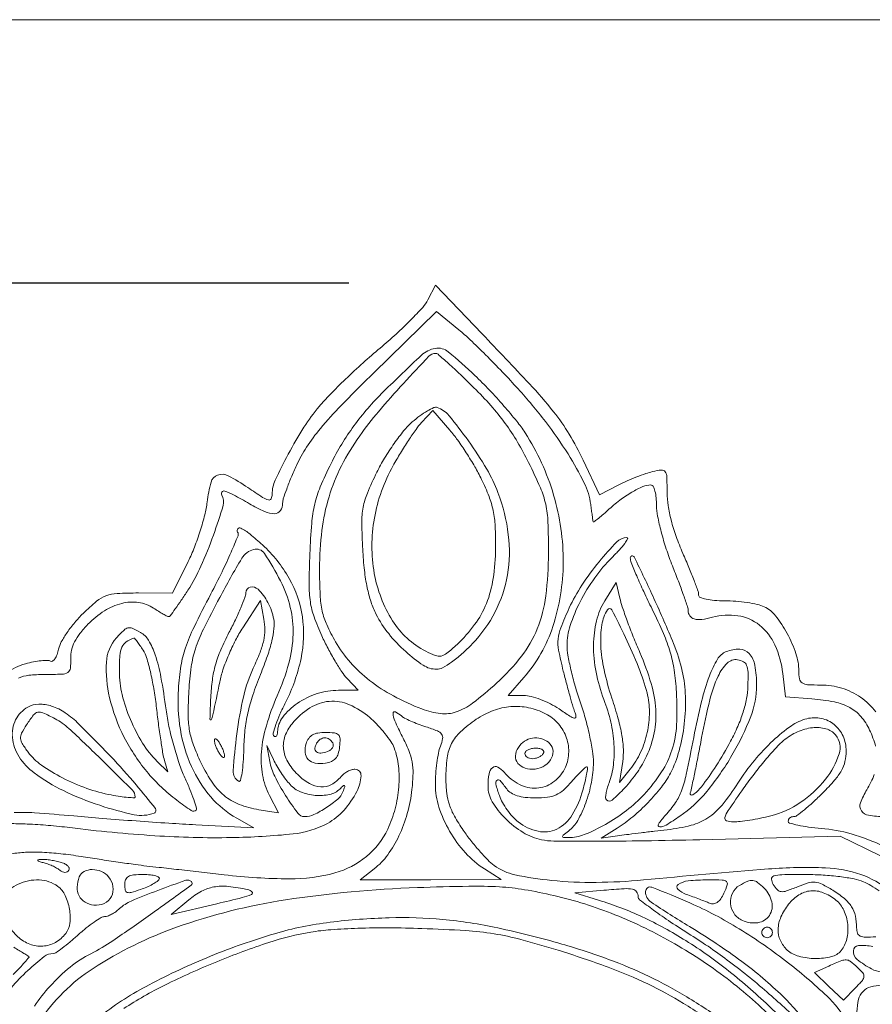
# Model space of a CAD drawing. Units: inches. Extents: x 2656 to 9931, y 1941 to 3068.
# Tile 40 of 46: x 2842.88 to 2854.27, y 2981.19 to 2994.35. Entities that reach past the tile are written whole.
import ezdxf

# ---------------------------------------------------------------- set-up
doc = ezdxf.new("R2010")
doc.units = ezdxf.units.IN
for name, color, linetype, lineweight in [('A-ANNO-DIMS', 2, 'Continuous', 18), ('A-ELEV-FNSH', 8, 'Continuous', 13), ('A-ELEV-ORN', 8, 'Continuous', 13)]:
    doc.layers.add(name, color=color, linetype=linetype, lineweight=lineweight)
doc.styles.get("Standard").update_dxf_attribs({"font": 'arial.ttf'})
doc.dimstyles.new('ISO-25', dxfattribs={"dimtxt": 6, "dimasz": 2.5, "dimexe": 1.25, "dimexo": 0.625, "dimtad": 1, "dimdec": 0, "dimlunit": 3, "dimtxsty": 'Standard', "dimcen": 2.5, "dimadec": 0, "dimazin": 0, "dimtfac": 1, "dimtdec": 0, "dimtmove": 0, "dimatfit": 3, "dimfxl": 1, "dimarcsym": 0})

# ---------------------------------------------------------------- blocks, each defined once
blk = doc.blocks.new('*D152')
at = {"layer": 'A-ANNO-DIMS', "color": 0, "lineweight": -2, "transparency": 16777216}
for p, q in [((2847.28, 2990.828), (2707.323, 2990.828)), ((2708.573, 2988.328), (2708.573, 2952.971)), ((2847.248, 2950.471), (2707.323, 2950.471))]:
    blk.add_line(p, q, dxfattribs=at)
at = {"layer": 'A-ANNO-DIMS', "color": 0, "transparency": 16777216}
for points in [[(2708.156, 2988.328), (2708.989, 2988.328), (2708.573, 2990.828)], [(2708.156, 2952.971), (2708.989, 2952.971), (2708.573, 2950.471)]]:
    blk.add_solid(points, dxfattribs=at)
at = {"layer": 'Defpoints', "color": 0, "transparency": 16777216}
for p in [(2847.905, 2990.828), (2708.573, 2950.471), (2847.873, 2950.471)]:
    blk.add_point(p, dxfattribs=at)
at = {"layer": 'A-ANNO-DIMS', "color": 0, "transparency": 16777216, "insert": (2704.843, 2970.649), "char_height": 6, "attachment_point": 5, "rotation": 90}
blk.add_mtext('3\'-4 1/2"', dxfattribs=at)
blk = doc.blocks.new('*D153')
at = {"layer": 'A-ANNO-DIMS', "color": 0, "lineweight": -2, "transparency": 16777216}
for p, q in [((2826.64, 2993.722), (2826.64, 2703.709)), ((2829.546, 2956.424), (2829.546, 2703.709)), ((2824.14, 2704.959), (2821.64, 2704.959)), ((2826.64, 2704.959), (2829.546, 2704.959)), ((2832.046, 2704.959), (2851.745, 2704.959))]:
    blk.add_line(p, q, dxfattribs=at)
at = {"layer": 'A-ANNO-DIMS', "color": 0, "transparency": 16777216}
for points in [[(2824.14, 2705.376), (2824.14, 2704.543), (2826.64, 2704.959)], [(2832.046, 2705.376), (2832.046, 2704.543), (2829.546, 2704.959)]]:
    blk.add_solid(points, dxfattribs=at)
at = {"layer": 'Defpoints', "color": 0, "transparency": 16777216}
for p in [(2826.64, 2994.347), (2829.546, 2957.049), (2829.546, 2704.959)]:
    blk.add_point(p, dxfattribs=at)
at = {"layer": 'A-ANNO-DIMS', "color": 0, "transparency": 16777216, "insert": (2843.145, 2708.65), "char_height": 6, "attachment_point": 5}
blk.add_mtext('0\'-3"', dxfattribs=at)
blk = doc.blocks.new('*D154')
at = {"layer": 'A-ANNO-DIMS', "color": 0, "lineweight": -2, "transparency": 16777216}
for p, q in [((2708.573, 2996.847), (2708.573, 2999.347)), ((2826.015, 2994.347), (2707.323, 2994.347)), ((2708.573, 2994.347), (2708.573, 2990.828)), ((2847.28, 2990.828), (2707.323, 2990.828)), ((2708.573, 2988.328), (2708.573, 2954.647))]:
    blk.add_line(p, q, dxfattribs=at)
at = {"layer": 'A-ANNO-DIMS', "color": 0, "transparency": 16777216}
for points in [[(2708.156, 2996.847), (2708.989, 2996.847), (2708.573, 2994.347)], [(2708.156, 2988.328), (2708.989, 2988.328), (2708.573, 2990.828)]]:
    blk.add_solid(points, dxfattribs=at)
at = {"layer": 'Defpoints', "color": 0, "transparency": 16777216}
for p in [(2826.64, 2994.347), (2708.573, 2990.828), (2847.905, 2990.828)]:
    blk.add_point(p, dxfattribs=at)
at = {"layer": 'A-ANNO-DIMS', "color": 0, "transparency": 16777216, "insert": (2704.843, 2970.237), "char_height": 6, "attachment_point": 5, "rotation": 90}
blk.add_mtext('0\'-3 1/2"', dxfattribs=at)

msp = doc.modelspace()

# ---------------------------------------------------------------- linework, layer by layer
at = {"layer": 'A-ELEV-FNSH'}
msp.add_lwpolyline([(2826.64, 2994.347), (2868.226, 2994.347), (2868.226, 2892.035), (2826.64, 2892.035)], close=True, dxfattribs=at)
at = {"layer": 'A-ELEV-ORN'}
for points in [[(2854.315, 2985.099, 0.078135), (2854.113, 2985.294, 0.079077), (2853.862, 2985.416, 0.074196), (2853.581, 2985.458, -0.014444), (2853.405, 2985.463, -0.128754), (2853.332, 2985.487, -0.206552), (2853.297, 2985.539, -0.046553), (2853.287, 2985.647, 0.081788), (2853.249, 2985.878, 0.042113), (2853.132, 2986.146, 0.041941), (2852.978, 2986.382, 0.120789), (2852.825, 2986.503, 0.050427), (2852.733, 2986.534, 0.018265), (2852.597, 2986.56, 0.017897), (2852.445, 2986.578, 0.020342), (2852.299, 2986.584, -0.018674), (2852.16, 2986.589, -0.035131), (2852.048, 2986.605, -0.042536), (2851.971, 2986.629, -0.305397), (2851.95, 2986.66, 0.085772), (2851.942, 2986.71, 0.004985), (2851.888, 2986.855, 0.007447), (2851.82, 2987.027, 0.005403), (2851.739, 2987.217, -0.017471), (2851.649, 2987.443, -0.022274), (2851.583, 2987.659, -0.024666), (2851.542, 2987.856, -0.039017), (2851.528, 2988.027, 0.008441), (2851.525, 2988.241, 0.142371), (2851.503, 2988.308, 0.273929), (2851.454, 2988.331, 0.034912), (2851.335, 2988.31, 0.024588), (2851.243, 2988.283, 0.010575), (2851.122, 2988.238, 0.010434), (2850.996, 2988.185, 0.013571), (2850.883, 2988.131), (2850.624, 2987.998), (2850.407, 2988.462, 0.026394), (2850.221, 2988.808, 0.032728), (2850.012, 2989.109, 0.019173), (2849.69, 2989.482, 0.003433), (2849.057, 2990.151), (2848.435, 2990.799), (2848.335, 2990.605, -0.064322), (2848.264, 2990.503, -0.01162), (2848.105, 2990.336, -0.012355), (2847.909, 2990.147, -0.010908), (2847.695, 2989.96, 0.00918), (2847.469, 2989.763, 0.007525), (2847.234, 2989.545, 0.007613), (2847.024, 2989.337, 0.019853), (2846.881, 2989.18, 0.032915), (2846.679, 2988.903, 0.018495), (2846.469, 2988.543, 0.015337), (2846.295, 2988.194, 0.10597), (2846.254, 2988.008, -0.116612), (2846.239, 2987.947, -0.354776), (2846.203, 2987.931, -0.077717), (2846.127, 2987.965, -0.005231), (2845.93, 2988.096, 0.027818), (2845.667, 2988.253, 0.209245), (2845.526, 2988.264, 0.245289), (2845.437, 2988.168, 0.037684), (2845.385, 2987.903, -0.03191), (2845.354, 2987.732, -0.0157), (2845.293, 2987.518, -0.01551), (2845.216, 2987.3, -0.021792), (2845.133, 2987.11), (2844.924, 2986.686), (2844.467, 2986.688, 0.013726), (2844.183, 2986.681, 0.075832), (2844.034, 2986.65, 0.085147), (2843.909, 2986.578, 0.019712), (2843.728, 2986.414, 0.025371), (2843.617, 2986.294, 0.023836), (2843.516, 2986.161, 0.024569), (2843.438, 2986.035, 0.071714), (2843.402, 2985.939, -0.032608), (2843.381, 2985.865, -0.059736), (2843.352, 2985.809, -0.094985), (2843.322, 2985.778, -0.298499), (2843.295, 2985.777, 0.144064), (2843.255, 2985.788, 0.021126), (2843.17, 2985.783, 0.022408), (2843.067, 2985.768, 0.017548), (2842.958, 2985.742, 0.091949), (2842.702, 2985.62, 0.038622)], [(2842.866, 2985.551, -0.083292), (2843.002, 2985.588, -0.025328), (2843.215, 2985.599, 0.00912), (2843.445, 2985.603, 0.128792), (2843.524, 2985.627, 0.230001), (2843.559, 2985.682, 0.036545), (2843.565, 2985.813, -0.063476), (2843.576, 2985.925, -0.05995), (2843.615, 2986.034, -0.049883), (2843.686, 2986.146, -0.026445), (2843.794, 2986.27, -0.057798), (2844.014, 2986.449, -0.082041), (2844.245, 2986.549, -0.095324), (2844.469, 2986.561, -0.11109), (2844.669, 2986.486, 0.007454), (2844.737, 2986.443, 0.010398), (2844.8, 2986.406, 0.007107), (2844.853, 2986.377, 0.120632), (2844.872, 2986.373, 0.235905), (2844.89, 2986.382, 0.003736), (2844.96, 2986.476, 0.008958), (2845.039, 2986.59, 0.005707), (2845.128, 2986.724, 0.036676), (2845.302, 2987.046, 0.020464), (2845.469, 2987.459, 0.013319), (2845.599, 2987.859, 0.213754), (2845.581, 2987.997, -0.305446), (2845.583, 2988.037, -0.321124), (2845.62, 2988.05, -0.047856), (2845.739, 2987.999, -0.008628), (2845.949, 2987.881, 0.025918), (2846.153, 2987.776, 0.110206), (2846.287, 2987.747, 0.24323), (2846.363, 2987.788, 0.152107), (2846.394, 2987.887, -0.078541), (2846.403, 2987.947, -0.008908), (2846.448, 2988.076, -0.010604), (2846.507, 2988.23, -0.008438), (2846.578, 2988.393, -0.040004), (2846.712, 2988.635, -0.027614), (2846.899, 2988.886, -0.019052), (2847.176, 2989.193, -0.006251), (2847.606, 2989.624), (2848.45, 2990.448), (2848.749, 2990.203, -0.01845), (2848.897, 2990.072, -0.006117), (2849.105, 2989.87, -0.006081), (2849.329, 2989.64, -0.006877), (2849.539, 2989.414, -0.019396), (2849.903, 2988.978, -0.023978), (2850.205, 2988.545, -0.025885), (2850.422, 2988.156, -0.081827), (2850.508, 2987.871, 0.000371), (2850.518, 2987.794, 0.000496), (2850.528, 2987.723, 0.000342), (2850.536, 2987.664, 0.00521), (2850.539, 2987.643, 0.548711), (2850.549, 2987.639, 0.013408), (2850.599, 2987.674, 0.016834), (2850.662, 2987.726, 0.009167), (2850.737, 2987.793, -0.025193), (2850.895, 2987.926, -0.02965), (2851.057, 2988.034, -0.031965), (2851.205, 2988.109, -0.101207), (2851.313, 2988.131, -0.284785), (2851.342, 2988.113, -0.049006), (2851.366, 2988.05, -0.040655), (2851.382, 2987.961, -0.025665), (2851.388, 2987.855, 0.049109), (2851.402, 2987.714, 0.015173), (2851.45, 2987.505, 0.015015), (2851.518, 2987.274, 0.015963), (2851.599, 2987.052, -0.004381), (2851.679, 2986.845, -0.006165), (2851.748, 2986.659, -0.003777), (2851.802, 2986.501, -0.081071), (2851.81, 2986.453, 0.155966), (2851.832, 2986.382, 0.172026), (2851.891, 2986.341, 0.10107), (2851.991, 2986.334, 0.034921), (2852.134, 2986.363, -0.105391), (2852.473, 2986.384, -0.132014), (2852.762, 2986.259, -0.119243), (2852.969, 2985.993, -0.076479), (2853.074, 2985.614), (2853.111, 2985.3), (2853.462, 2985.273, -0.029523), (2853.762, 2985.232, -0.074901), (2853.968, 2985.158, -0.093016), (2854.116, 2985.038, -0.065621), (2854.233, 2984.857, -0.044451), (2854.313, 2984.64, -0.078218)], [(2854.424, 2983.306, 0.034451), (2853.986, 2983.469, 0.051823), (2853.586, 2983.543, -0.012852), (2853.418, 2983.561, -0.020808), (2853.275, 2983.586, -0.016013), (2853.165, 2983.614, -0.33473), (2853.146, 2983.639, -0.118163), (2853.152, 2983.662, -0.100614), (2853.167, 2983.682, -0.092537), (2853.191, 2983.695, -0.082719), (2853.218, 2983.7, 0.160905), (2853.261, 2983.714, 0.011177), (2853.362, 2983.792, 0.014973), (2853.479, 2983.894, 0.010663), (2853.605, 2984.015, 0.016588), (2853.766, 2984.187, 0.052031), (2853.857, 2984.316, 0.071324), (2853.904, 2984.437, 0.056637), (2853.92, 2984.576, 0.103225), (2853.878, 2984.775, 0.118359), (2853.761, 2984.93, 0.1216), (2853.589, 2985.012, 0.112975), (2853.394, 2985.008, 0.091427), (2853.188, 2984.914, 0.035379), (2852.943, 2984.715, 0.032673), (2852.695, 2984.451, 0.029758), (2852.475, 2984.149, -0.028189), (2852.263, 2983.855, -0.076789), (2852.074, 2983.684, -0.082317), (2851.85, 2983.584, -0.035894), (2851.528, 2983.525, 0.001697), (2851.362, 2983.506, 0.001346), (2851.183, 2983.484, 0.00136), (2851.017, 2983.463, 0.003403), (2850.895, 2983.447), (2850.649, 2983.412), (2850.86, 2983.546, 0.032786), (2851.07, 2983.699, 0.026073), (2851.276, 2983.89, 0.026722), (2851.452, 2984.093, 0.046509), (2851.573, 2984.281, 0.053502), (2851.689, 2984.58, 0.036945), (2851.758, 2984.938, 0.036528), (2851.773, 2985.307, 0.047498), (2851.731, 2985.643, 0.042706), (2851.615, 2986.012, 0.009719), (2851.353, 2986.613, 0.007724), (2851.088, 2987.169, 0.786926), (2851.037, 2987.157, 0.098595), (2851.049, 2987.096, 0.005676), (2851.122, 2986.917, 0.008467), (2851.216, 2986.706, 0.00611), (2851.328, 2986.473, -0.012354), (2851.48, 2986.145, -0.031365), (2851.57, 2985.898, -0.035368), (2851.622, 2985.659, -0.019934), (2851.653, 2985.365, -0.029859), (2851.655, 2984.925, -0.062769), (2851.593, 2984.589, -0.068214), (2851.455, 2984.297, -0.041404), (2851.22, 2983.995, -0.043392), (2850.988, 2983.783, -0.033937), (2850.704, 2983.595, -0.034654), (2850.423, 2983.46, -0.09505), (2850.208, 2983.419, -0.016241), (2850.143, 2983.421, -0.40699), (2850.132, 2983.433, -0.217056), (2850.142, 2983.452, -0.007438), (2850.211, 2983.507, 0.104056), (2850.334, 2983.648, 0.040712), (2850.442, 2983.884, 0.0392), (2850.518, 2984.158, 0.04772), (2850.544, 2984.424, 0.039125), (2850.532, 2984.576, 0.014351), (2850.492, 2984.788, 0.014125), (2850.435, 2985.019, 0.016453), (2850.368, 2985.234, -0.01367), (2850.3, 2985.445, -0.013019), (2850.244, 2985.663, -0.01308), (2850.203, 2985.858, -0.044292), (2850.192, 2985.987, -0.079543), (2850.235, 2986.253, -0.038926), (2850.367, 2986.571, -0.037036), (2850.562, 2986.89, -0.041614), (2850.794, 2987.164, 0.012038), (2850.891, 2987.265, 0.024408), (2850.962, 2987.35, 0.032837), (2851.001, 2987.411, 0.572992), (2850.992, 2987.428, 0.203102), (2850.857, 2987.371, 0.020739), (2850.621, 2987.106, 0.026278), (2850.389, 2986.791, 0.038243), (2850.222, 2986.489, 0.01216), (2850.108, 2986.222, 0.071457), (2850.073, 2986.075, 0.072281), (2850.08, 2985.924, 0.012602), (2850.142, 2985.645, 0.003624), (2850.188, 2985.47, 0.004047), (2850.233, 2985.302, 0.003736), (2850.275, 2985.159, 0.021333), (2850.301, 2985.085, -0.093964), (2850.311, 2985.032, -0.486856), (2850.291, 2985.016, -0.082498), (2850.231, 2985.042, -0.006579), (2850.086, 2985.138, 0.031762), (2849.969, 2985.207, 0.026558), (2849.837, 2985.265, 0.027385), (2849.711, 2985.305, 0.063462), (2849.612, 2985.318), (2849.404, 2985.318), (2849.615, 2985.558, 0.101844), (2850.003, 2986.241, 0.077512), (2850.141, 2987.092, 0.072839), (2850.013, 2987.996, 0.072078), (2849.632, 2988.829, 0.026422), (2849.52, 2988.983, 0.010022), (2849.349, 2989.186, 0.009893), (2849.154, 2989.4, 0.01192), (2848.962, 2989.593, 0.018391), (2848.606, 2989.91, 0.219576), (2848.432, 2989.956, 0.145576), (2848.247, 2989.864, 0.006907), (2847.743, 2989.379, 0.01889), (2847.531, 2989.153, 0.021022), (2847.345, 2988.92, 0.021463), (2847.183, 2988.676, 0.021586), (2847.042, 2988.42, 0.014989), (2846.897, 2988.105, 0.041973), (2846.822, 2987.874, 0.03764), (2846.782, 2987.619, 0.010219), (2846.757, 2987.213, 0.008108), (2846.747, 2986.804, 0.038176), (2846.764, 2986.569, 0.050177), (2846.813, 2986.371, 0.020973), (2846.917, 2986.115, 0.013565), (2847, 2985.947, 0.012733), (2847.094, 2985.779, 0.012815), (2847.184, 2985.635, 0.042128), (2847.254, 2985.546), (2847.403, 2985.388), (2847.14, 2985.388, 0.07865), (2846.855, 2985.343, 0.071598), (2846.588, 2985.212, 0.079818), (2846.395, 2985.028, 0.158524), (2846.326, 2984.831, -0.047162), (2846.322, 2984.796, -0.134812), (2846.31, 2984.775, -0.251455), (2846.295, 2984.769, -0.15697), (2846.277, 2984.778, -0.271092), (2846.267, 2984.814, -0.01545), (2846.303, 2984.929, -0.020165), (2846.358, 2985.069, -0.01311), (2846.433, 2985.225, 0.065004), (2846.639, 2985.812, 0.088793), (2846.657, 2986.371, 0.092884), (2846.481, 2986.882, 0.078127), (2846.124, 2987.331, 0.016395), (2845.958, 2987.474, 0.049956), (2845.834, 2987.555, 0.368564), (2845.795, 2987.546, 0.306498), (2845.793, 2987.502, -0.23943), (2845.798, 2987.452, -0.005733), (2845.705, 2987.232, -0.011318), (2845.585, 2986.972, -0.007294), (2845.435, 2986.676, 0.007423), (2845.21, 2986.232, 0.031468), (2845.097, 2985.957, 0.042853), (2845.036, 2985.714, 0.022925), (2845.002, 2985.405, 0.056615), (2845.028, 2984.863, 0.065886), (2845.177, 2984.369, 0.071367), (2845.435, 2983.964, 0.08766), (2845.781, 2983.679), (2846.007, 2983.552), (2845.233, 2983.592, -0.003395), (2844.876, 2983.612, -0.00184), (2844.436, 2983.642, -0.001832), (2843.989, 2983.676, -0.002895), (2843.606, 2983.709, 0.005241), (2843.08, 2983.751, 0.032074), (2842.808, 2983.753, 0.046774)], [(2842.742, 2983.607, -0.010086), (2842.983, 2983.601, -0.010454), (2843.264, 2983.583, -0.009794), (2843.55, 2983.553, 0.014603), (2844.689, 2983.445, 0.020573), (2845.709, 2983.42, 0.021554), (2846.535, 2983.469, 0.098726), (2846.992, 2983.61, 0.086544), (2847.211, 2983.783, 0.064842), (2847.385, 2984.037, 0.105005), (2847.441, 2984.247, 0.429394), (2847.36, 2984.333, 0.076994), (2847.314, 2984.326, 0.044443), (2847.262, 2984.304, 0.043169), (2847.213, 2984.273, 0.055175), (2847.174, 2984.235, -0.094539), (2847.045, 2984.129, -0.137453), (2846.903, 2984.096, -0.121204), (2846.751, 2984.141, -0.064485), (2846.595, 2984.261, -0.062539), (2846.462, 2984.433, -0.106068), (2846.405, 2984.604, -0.115654), (2846.425, 2984.774, -0.084243), (2846.519, 2984.939, -0.078947), (2846.757, 2985.152, -0.123459), (2847.016, 2985.24, -0.122999), (2847.287, 2985.195, -0.078015), (2847.559, 2985.023, -0.023138), (2847.662, 2984.924, -0.02043), (2847.759, 2984.812, -0.020932), (2847.839, 2984.703, -0.056713), (2847.883, 2984.619, -0.065298), (2847.941, 2984.376, -0.046), (2847.945, 2984.096, -0.044024), (2847.896, 2983.805, -0.046139), (2847.797, 2983.533, -0.111372), (2847.513, 2983.167, -0.104185), (2847.092, 2982.948, -0.070935), (2846.484, 2982.868, -0.025816), (2845.614, 2982.922, 0.000041), (2845.311, 2982.957, 0.000041), (2845.008, 2982.992, 0.00004), (2844.743, 2983.022, 0.000159), (2844.58, 2983.04, -0.005888), (2844.426, 2983.06, -0.001908), (2844.198, 2983.092, -0.001902), (2843.945, 2983.13, -0.002136), (2843.701, 2983.168, 0.013188), (2843.43, 2983.204, 0.017307), (2843.181, 2983.223, 0.019272), (2842.96, 2983.223, 0.031038), (2842.772, 2983.203, -0.002177)], [(2854.502, 2982.71, 0.090302), (2854.115, 2982.926, 0.071489), (2853.644, 2983.015, 0.030983), (2852.881, 2983.001, 0.003778), (2851.212, 2982.854, -0.021814), (2850.58, 2982.821, -0.026279), (2849.987, 2982.847, -0.027515), (2849.496, 2982.923, -0.109001), (2849.219, 2983.048, -0.039008), (2849.134, 2983.122, -0.013678), (2849.023, 2983.242, -0.013486), (2848.908, 2983.38, -0.015368), (2848.806, 2983.519, -0.021273), (2848.689, 2983.706, -0.047989), (2848.621, 2983.858, -0.052132), (2848.586, 2984.013, -0.029551), (2848.574, 2984.205, -0.032073), (2848.592, 2984.486, -0.085895), (2848.651, 2984.678, -0.089345), (2848.77, 2984.834, -0.036649), (2848.979, 2985, -0.05968), (2849.206, 2985.117, -0.069858), (2849.442, 2985.17, -0.071671), (2849.679, 2985.155, -0.067725), (2849.906, 2985.074, -0.096375), (2850.077, 2984.939, -0.095623), (2850.185, 2984.75, -0.097447), (2850.213, 2984.537, -0.104526), (2850.158, 2984.335, -0.120644), (2850, 2984.154, -0.141327), (2849.786, 2984.08, -0.132721), (2849.555, 2984.13, -0.100833), (2849.352, 2984.293, 0.099524), (2849.267, 2984.362, 0.306948), (2849.198, 2984.354, 0.175194), (2849.15, 2984.27, 0.041792), (2849.137, 2984.109, 0.134004), (2849.194, 2983.899, 0.062873), (2849.368, 2983.674, 0.060359), (2849.605, 2983.488, 0.086765), (2849.852, 2983.391, 0.047774), (2850.015, 2983.374, 0.002239), (2850.569, 2983.372, 0.003679), (2851.228, 2983.377, 0.002634), (2851.964, 2983.392), (2853.842, 2983.44), (2854.371, 2983.182, -0.01869)], [(2854.296, 2984.264, -0.046304), (2854.196, 2984.059, 0.047957), (2854.111, 2983.884, 0.239863), (2854.123, 2983.779, 0.210398), (2854.218, 2983.718, 0.03751), (2854.433, 2983.701, -0.076239)], [(2854.317, 2982.096, -0.017844), (2854.177, 2982.089, -0.111032), (2854.108, 2982.103, -0.203959), (2854.072, 2982.142, -0.084493), (2854.06, 2982.213, 0.053126), (2854.043, 2982.372, 0.088219), (2853.992, 2982.496, 0.078617), (2853.897, 2982.605, 0.034796), (2853.741, 2982.717, 0.021635), (2853.599, 2982.796, 0.093332), (2853.506, 2982.823, 0.097889), (2853.412, 2982.814, 0.025071), (2853.268, 2982.762, -0.014374), (2853.124, 2982.707, -0.11002), (2853.053, 2982.698, -0.177871), (2853.001, 2982.723, -0.052147), (2852.946, 2982.794, -0.128312), (2852.923, 2982.866, -0.345735), (2852.953, 2982.907, -0.067863), (2853.061, 2982.924, -0.004017), (2853.394, 2982.926, -0.016087), (2853.614, 2982.919, -0.015606), (2853.835, 2982.898, -0.015762), (2854.028, 2982.867, -0.053298), (2854.15, 2982.83, -0.033959), (2854.25, 2982.779, -0.019972), (2854.361, 2982.707, -0.019921)], [(2842.766, 2981.414, -0.024978), (2842.99, 2981.643, -0.020758), (2843.209, 2981.829, -0.166976), (2843.332, 2981.871, 0.152907), (2843.366, 2981.882, 0.009354), (2843.451, 2981.944, 0.013229), (2843.552, 2982.023, 0.009364), (2843.66, 2982.117, -0.013871), (2843.77, 2982.212, -0.01812), (2843.877, 2982.291, -0.015858), (2843.968, 2982.351, -0.136675), (2844.015, 2982.364, 0.09123), (2844.054, 2982.371, 0.031745), (2844.108, 2982.395, 0.030285), (2844.164, 2982.43, 0.030912), (2844.215, 2982.471, -0.082228), (2844.372, 2982.572, -0.011888), (2844.725, 2982.714, -0.006268), (2845.099, 2982.849, -0.287599), (2845.175, 2982.832, -0.460996), (2845.172, 2982.784, -0.001493), (2844.628, 2982.392, -0.006319), (2844.125, 2982.041, -0.032689), (2843.833, 2981.869, 0.054333), (2843.557, 2981.69, 0.037267), (2843.287, 2981.434, 0.03621), (2843.078, 2981.168, 0.154288)], [(2843.141, 2980.957, -0.10364), (2843.864, 2981.673, -0.058168), (2844.978, 2982.222, -0.047464), (2846.434, 2982.588, -0.029352), (2848.193, 2982.752, -0.004362), (2848.88, 2982.77, -0.01877), (2849.289, 2982.762, -0.026526), (2849.624, 2982.724, -0.016022), (2850.016, 2982.646, -0.038715), (2850.832, 2982.389, -0.034771), (2851.63, 2982.001, -0.034471), (2852.373, 2981.502, -0.036376), (2853.026, 2980.915, 0.00697)], [(2853.43, 2980.888, 0.039762), (2853.073, 2981.299, 0.035403), (2852.526, 2981.765, 0.022219), (2851.827, 2982.232, -0.010114), (2851.315, 2982.557, -0.257227), (2851.241, 2982.699, -0.51849), (2851.326, 2982.756, -0.012975), (2851.834, 2982.547, -0.034146), (2852.492, 2982.201, -0.0272), (2853.15, 2981.743, -0.027027), (2853.697, 2981.268, -0.092556), (2853.968, 2980.885, 0.014479)], [(2852.297, 2980.956, 0.020948), (2851.793, 2981.291, 0.02459), (2851.288, 2981.564, 0.02374), (2850.745, 2981.793, 0.017347), (2850.122, 2981.998, 0.017713), (2849.266, 2982.213, 0.029402), (2848.532, 2982.326, 0.031017), (2847.817, 2982.349, 0.022786), (2847.027, 2982.289, 0.041752), (2846.286, 2982.136, 0.024654), (2845.432, 2981.836, 0.024644), (2844.611, 2981.454, 0.041345), (2843.97, 2981.045, 0.012422)], [(2844.271, 2981.135, -0.0302), (2844.821, 2981.45, -0.01769), (2845.514, 2981.762, -0.017702), (2846.211, 2982.019, -0.037526), (2846.77, 2982.157, -0.023556), (2847.037, 2982.189, -0.010004), (2847.398, 2982.208, -0.009217), (2847.812, 2982.214, -0.007701), (2848.253, 2982.205, -0.007144), (2848.836, 2982.177, -0.023875), (2849.217, 2982.134, -0.025809), (2849.576, 2982.058, -0.009462), (2850.075, 2981.914, -0.013133), (2850.741, 2981.688, -0.023644), (2851.272, 2981.464, -0.025775), (2851.747, 2981.205, -0.019692), (2852.24, 2980.876, -0.007963)], [(2842.804, 2981.955, 0.000076), (2842.874, 2981.911, 0.000108), (2842.936, 2981.873, 0.000061), (2842.989, 2981.84, 0.001532), (2843.003, 2981.831, -0.455409), (2843.005, 2981.819, -0.005577), (2842.951, 2981.755, -0.011717), (2842.882, 2981.678, -0.006865), (2842.795, 2981.589, -0.020091)], [(2854.528, 2981.626, -0.173005), (2854.26, 2981.665, -0.048254), (2854.067, 2981.792, -0.240913), (2854.016, 2981.906, -0.374645), (2854.084, 2981.976, -0.070536), (2854.276, 2981.965, 0.042314)], [(2854.063, 2981.092, -0.053592), (2854.085, 2981.259, -0.136805), (2854.145, 2981.365, -0.127241), (2854.248, 2981.426, -0.071275), (2854.394, 2981.446, -0.065833)]]:
    msp.add_lwpolyline(points, format="xyb", dxfattribs=at)
for points in [[(2848.949, 2989.431, -0.017705), (2849.174, 2989.192, -0.022163), (2849.365, 2988.954, -0.022708), (2849.53, 2988.705, -0.020336), (2849.679, 2988.432, -0.012444), (2849.836, 2988.093, -0.048338), (2849.907, 2987.873, -0.044828), (2849.937, 2987.635, -0.009686), (2849.944, 2987.22, -0.031328), (2849.907, 2986.648, -0.063117), (2849.794, 2986.211, -0.069293), (2849.584, 2985.842, -0.04557), (2849.251, 2985.483, -0.019387), (2848.931, 2985.217, -0.080794), (2848.71, 2985.098, -0.114651), (2848.505, 2985.077, -0.060196), (2848.254, 2985.139, -0.031621), (2847.874, 2985.313, -0.042292), (2847.556, 2985.519, -0.046038), (2847.299, 2985.76, -0.051489), (2847.101, 2986.035, -0.022207), (2846.983, 2986.265, -0.053988), (2846.922, 2986.445, -0.043412), (2846.895, 2986.657, -0.010375), (2846.887, 2987.012, -0.030913), (2846.918, 2987.524, -0.042839), (2847.013, 2987.973, -0.044516), (2847.179, 2988.386, -0.037558), (2847.424, 2988.789, -0.019818), (2847.674, 2989.11, -0.010653), (2848.006, 2989.487, -0.004218), (2848.347, 2989.851, -0.20536), (2848.437, 2989.889, -0.181057), (2848.469, 2989.877, -0.00329), (2848.608, 2989.755, -0.007702), (2848.768, 2989.607, -0.005012)], [(2848.125, 2988.973, 0.041366), (2848.013, 2988.857, 0.017676), (2847.883, 2988.685, 0.017347), (2847.756, 2988.491, 0.021841), (2847.652, 2988.302, 0.015479), (2847.526, 2988.023, 0.053533), (2847.469, 2987.833, 0.048234), (2847.451, 2987.625, 0.010916), (2847.463, 2987.271, 0.013767), (2847.486, 2986.991, 0.023714), (2847.523, 2986.759, 0.028229), (2847.575, 2986.566, 0.039754), (2847.644, 2986.401, 0.05001), (2847.81, 2986.145, 0.03921), (2848.037, 2985.904, 0.039535), (2848.272, 2985.722, 0.145915), (2848.449, 2985.669, 0.125304), (2848.53, 2985.69, 0.029667), (2848.649, 2985.765, 0.027356), (2848.786, 2985.873, 0.019289), (2848.927, 2986.009, 0.073793), (2849.232, 2986.436, 0.076247), (2849.396, 2986.929, 0.072747), (2849.408, 2987.467, 0.058947), (2849.27, 2988.029, 0.044539), (2849.12, 2988.343, 0.021074), (2848.874, 2988.72, 0.016594), (2848.614, 2989.059, 0.142094), (2848.458, 2989.166, 0.186611), (2848.412, 2989.164, 0.027261), (2848.327, 2989.121, 0.027725), (2848.227, 2989.055, 0.020547)], [(2849.05, 2988.206, -0.021855), (2849.15, 2987.979, -0.042029), (2849.205, 2987.789, -0.037924), (2849.232, 2987.58, -0.014668), (2849.238, 2987.287, -0.03482), (2849.205, 2986.88, -0.058125), (2849.116, 2986.549, -0.062666), (2848.958, 2986.265, -0.048569), (2848.723, 2986, -0.016192), (2848.587, 2985.883, -0.117547), (2848.511, 2985.846, -0.144734), (2848.433, 2985.852, -0.028801), (2848.304, 2985.91, -0.134355), (2847.861, 2986.318, -0.09671), (2847.618, 2986.95, -0.087319), (2847.619, 2987.686, -0.083772), (2847.869, 2988.389, -0.009605), (2847.968, 2988.558, -0.009005), (2848.075, 2988.727, -0.009012), (2848.175, 2988.873, -0.030344), (2848.248, 2988.964), (2848.398, 2989.128), (2848.628, 2988.862, -0.023773), (2848.73, 2988.733, -0.011854), (2848.847, 2988.56, -0.011739), (2848.96, 2988.375, -0.01693)], [(2846.365, 2986.85, -0.05862), (2846.496, 2986.496, -0.066947), (2846.534, 2986.136, -0.060176), (2846.476, 2985.75, -0.036203), (2846.321, 2985.312, 0.031452), (2846.176, 2984.915, 0.052381), (2846.111, 2984.565, 0.062293), (2846.125, 2984.257, 0.076873), (2846.217, 2983.984), (2846.338, 2983.75), (2846.077, 2983.792, -0.053112), (2845.813, 2983.864, -0.08112), (2845.609, 2983.985, -0.07403), (2845.442, 2984.173, -0.037264), (2845.288, 2984.452, -0.02111), (2845.194, 2984.683, -0.046993), (2845.147, 2984.867, -0.040967), (2845.132, 2985.071, -0.012781), (2845.142, 2985.378, -0.01958), (2845.174, 2985.704, -0.045505), (2845.229, 2985.944, -0.035232), (2845.335, 2986.203, -0.007951), (2845.553, 2986.627, -0.011569), (2845.849, 2987.152, -0.193973), (2846.005, 2987.27, -0.324163), (2846.151, 2987.216, -0.027798)], [(2845.902, 2986.69, -0.090133), (2845.89, 2986.628, -0.009811), (2845.836, 2986.491, -0.011764), (2845.763, 2986.329, -0.009238), (2845.677, 2986.158, 0.019456), (2845.568, 2985.929, 0.032634), (2845.497, 2985.728, 0.034126), (2845.455, 2985.526, 0.023904), (2845.434, 2985.295, 0.003033), (2845.423, 2985, 0.7785), (2845.439, 2984.995, 0.08097), (2845.463, 2985.059, 0.000964), (2845.553, 2985.5, -0.033342), (2845.597, 2985.663, -0.017451), (2845.673, 2985.86, -0.017281), (2845.765, 2986.057, -0.025301), (2845.861, 2986.223), (2846.096, 2986.588), (2846.143, 2986.337, -0.047851), (2846.156, 2986.193, -0.051834), (2846.141, 2986.054, -0.040393), (2846.092, 2985.894, -0.016103), (2846.002, 2985.684, 0.053301), (2845.874, 2985.312, 0.024063), (2845.782, 2984.804, 0.015985), (2845.734, 2984.311, 0.278337), (2845.805, 2984.174, 0.503517), (2845.83, 2984.183, 0.02371), (2845.851, 2984.284, 0.023184), (2845.867, 2984.427, 0.01246), (2845.875, 2984.604, -0.022882), (2845.891, 2984.853, -0.027681), (2845.929, 2985.085, -0.025678), (2845.996, 2985.324, -0.015771), (2846.098, 2985.599, 0.012836), (2846.191, 2985.847, 0.025315), (2846.25, 2986.049, 0.031987), (2846.278, 2986.212, 0.071965), (2846.274, 2986.338, 0.072982), (2846.198, 2986.559, 0.08496), (2846.065, 2986.737, 0.256007), (2845.96, 2986.765, 0.344476)], [(2850.697, 2986.584, 0.080947), (2850.586, 2986.317, 0.055842), (2850.546, 2985.991, 0.05064), (2850.579, 2985.632, 0.042649), (2850.684, 2985.264, -0.034798), (2850.776, 2984.962, -0.040702), (2850.818, 2984.666, -0.044215), (2850.811, 2984.39, -0.062064), (2850.753, 2984.152, 0.022148), (2850.728, 2984.076, 0.030665), (2850.713, 2984.007, 0.031217), (2850.707, 2983.95, 0.206016), (2850.718, 2983.924, 0.393222), (2850.795, 2983.922, 0.02864), (2850.962, 2984.084, 0.03328), (2851.132, 2984.295, 0.044428), (2851.255, 2984.509, 0.058439), (2851.356, 2984.819, 0.065899), (2851.377, 2985.131, 0.056234), (2851.315, 2985.477, 0.029068), (2851.166, 2985.891, -0.006369), (2851.077, 2986.104, -0.006544), (2850.995, 2986.318, -0.00636), (2850.929, 2986.505, -0.027359), (2850.897, 2986.619), (2850.85, 2986.83)], [(2851.26, 2985.353, -0.065214), (2851.293, 2985.097, -0.054073), (2851.263, 2984.823, -0.053572), (2851.175, 2984.559, -0.061101), (2851.035, 2984.333), (2850.894, 2984.157), (2850.935, 2984.438, 0.046822), (2850.944, 2984.601, 0.032179), (2850.925, 2984.784, 0.02531), (2850.875, 2985.005, 0.012096), (2850.791, 2985.282, -0.025663), (2850.687, 2985.66, -0.04185), (2850.643, 2985.989, -0.051154), (2850.657, 2986.261, -0.099954), (2850.732, 2986.464, -0.581878), (2850.791, 2986.462, -0.009223), (2850.973, 2986.095, -0.01655), (2851.147, 2985.695, -0.029412)], [(2844.174, 2986.087, 0.172154), (2844.04, 2985.765, 0.071457), (2844.083, 2985.289, 0.061299), (2844.278, 2984.759, 0.055784), (2844.602, 2984.274, 0.030445), (2844.774, 2984.093, 0.024242), (2844.979, 2983.92, 0.016218), (2845.174, 2983.781, 0.357434), (2845.238, 2983.787, 0.279023), (2845.245, 2983.814, 0.008257), (2845.207, 2983.927, 0.014252), (2845.155, 2984.063, 0.009073), (2845.088, 2984.219, -0.026189), (2845.013, 2984.408, -0.013812), (2844.939, 2984.65, -0.013706), (2844.876, 2984.903, -0.020542), (2844.837, 2985.126, 0.011953), (2844.768, 2985.565, 0.034959), (2844.692, 2985.861, 0.052725), (2844.604, 2986.056, 0.138047), (2844.494, 2986.162, 0.019078), (2844.382, 2986.217, 0.16317), (2844.327, 2986.222, 0.139123), (2844.276, 2986.193, 0.012602)], [(2844.53, 2985.925, -0.072616), (2844.577, 2985.825, -0.01487), (2844.627, 2985.637, -0.015364), (2844.672, 2985.412, -0.0139), (2844.706, 2985.178, 0.004271), (2844.734, 2984.945, 0.004996), (2844.766, 2984.724, 0.004436), (2844.795, 2984.538, 0.030229), (2844.817, 2984.448), (2844.861, 2984.298), (2844.718, 2984.438, -0.058565), (2844.524, 2984.682, -0.04017), (2844.361, 2984.996, -0.04022), (2844.25, 2985.331, -0.059423), (2844.213, 2985.639, -0.016262), (2844.22, 2985.851, -0.085274), (2844.247, 2985.964, -0.138013), (2844.304, 2986.034, -0.070648), (2844.405, 2986.086, -0.31492), (2844.415, 2986.083, -0.006173), (2844.449, 2986.041, -0.012411), (2844.487, 2985.988, -0.007711)], [(2852.318, 2985.904, 0.165424), (2852.202, 2985.804, 0.042576), (2852.094, 2985.579, 0.03085), (2851.989, 2985.24, 0.01187), (2851.884, 2984.758, -0.004218), (2851.784, 2984.263, -0.035106), (2851.721, 2984.043, -0.064087), (2851.641, 2983.889, -0.03207), (2851.506, 2983.718, 0.032911), (2851.413, 2983.6, 0.585663), (2851.43, 2983.565, 0.151652), (2851.514, 2983.586, 0.013225), (2851.7, 2983.707, 0.070327), (2852.057, 2984.035, 0.039471), (2852.395, 2984.52, 0.039624), (2852.645, 2985.036, 0.0932), (2852.724, 2985.455, 0.04232), (2852.701, 2985.722, 0.142454), (2852.625, 2985.879, 0.207068), (2852.498, 2985.937, 0.10069)], [(2852.607, 2985.445, -0.03794), (2852.589, 2985.276, -0.029771), (2852.544, 2985.096, -0.027125), (2852.473, 2984.906, -0.020589), (2852.376, 2984.707, -0.017432), (2852.183, 2984.378, -0.024362), (2851.987, 2984.1, -0.072868), (2851.874, 2983.991, -0.707506), (2851.838, 2984.016, 0.015846), (2851.859, 2984.103, 0.001992), (2851.899, 2984.291, 0.002341), (2851.944, 2984.516, 0.001941), (2851.99, 2984.755, -0.013973), (2852.099, 2985.259, -0.04764), (2852.21, 2985.576, -0.087896), (2852.331, 2985.75, -0.236693), (2852.47, 2985.796, -0.091197), (2852.548, 2985.77, -0.174607), (2852.591, 2985.721, -0.088585), (2852.609, 2985.631, -0.013427)], [(2842.99, 2985.163, 0.150682), (2842.828, 2984.993, 0.140741), (2842.784, 2984.756, 0.118986), (2842.873, 2984.5, 0.09113), (2843.076, 2984.283, 0.047148), (2843.466, 2984.047, 0.03133), (2843.951, 2983.851, 0.029184), (2844.412, 2983.726, 0.144139), (2844.677, 2983.747, 0.505083), (2844.694, 2983.808, 0.008532), (2844.437, 2984.124, 0.014242), (2844.098, 2984.503, 0.008445), (2843.673, 2984.937, 0.045857), (2843.491, 2985.087, 0.069431), (2843.308, 2985.177, 0.084935), (2843.137, 2985.203, 0.123164)], [(2843.355, 2985.008, -0.067699), (2843.539, 2984.878, -0.005874), (2843.955, 2984.481, -0.002811), (2844.387, 2984.054, -0.198928), (2844.424, 2983.963, -0.426413), (2844.413, 2983.951, -0.01023), (2844.33, 2983.957, -0.016119), (2844.227, 2983.968, -0.009459), (2844.104, 2983.989, -0.03958), (2843.78, 2984.077, -0.03311), (2843.453, 2984.218, -0.03433), (2843.172, 2984.388, -0.079387), (2842.996, 2984.56, -0.020214), (2842.915, 2984.677, -0.12579), (2842.893, 2984.746, -0.13582), (2842.908, 2984.814, -0.025008), (2842.974, 2984.927, -0.018278), (2843.067, 2985.058, -0.179078), (2843.124, 2985.094, -0.159807), (2843.193, 2985.087, -0.013801)], [(2847.98, 2985.045, 0.068851), (2848.021, 2985.016, 0.013641), (2848.104, 2984.977, 0.014209), (2848.203, 2984.936, 0.012792), (2848.307, 2984.9, -0.016005), (2848.46, 2984.845, -0.140058), (2848.517, 2984.802, -0.211156), (2848.53, 2984.744, -0.043005), (2848.501, 2984.641, 0.042878), (2848.475, 2984.55, 0.015421), (2848.453, 2984.418, 0.015166), (2848.438, 2984.271, 0.017397), (2848.434, 2984.129, 0.078277), (2848.481, 2983.826, 0.053409), (2848.624, 2983.506, 0.052411), (2848.835, 2983.216, 0.066536), (2849.088, 2983.002), (2849.313, 2982.858), (2848.371, 2982.857), (2847.43, 2982.856), (2847.617, 2983.003, 0.068721), (2847.797, 2983.189, 0.046574), (2847.947, 2983.443, 0.043279), (2848.059, 2983.742, 0.039834), (2848.121, 2984.064, 0.022084), (2848.135, 2984.274, 0.051136), (2848.123, 2984.431, 0.051223), (2848.079, 2984.582, 0.022226), (2847.991, 2984.773, -0.011889), (2847.892, 2984.978, -0.096537), (2847.868, 2985.08, -0.566329), (2847.899, 2985.1, -0.074818)], [(2853.778, 2984.791, -0.25773), (2853.826, 2984.538, -0.090134), (2853.644, 2984.2, -0.074143), (2853.307, 2983.888, -0.0883), (2852.912, 2983.71, -0.011429), (2852.776, 2983.679, -0.010081), (2852.633, 2983.653, -0.01018), (2852.504, 2983.635, -0.029989), (2852.414, 2983.63, -0.084474), (2852.322, 2983.645, -0.40285), (2852.3, 2983.688, -0.075006), (2852.345, 2983.781, -0.003121), (2852.553, 2984.083, -0.011443), (2852.69, 2984.269, -0.010427), (2852.84, 2984.456, -0.010498), (2852.98, 2984.616, -0.032945), (2853.084, 2984.716, -0.067963), (2853.27, 2984.833, -0.080185), (2853.47, 2984.888, -0.094887), (2853.65, 2984.874, -0.153097)], [(2846.708, 2984.678, 0.095719), (2846.694, 2984.555, 0.177301), (2846.735, 2984.465, 0.16002), (2846.828, 2984.416, 0.075231), (2846.966, 2984.415, 0.065371), (2847.045, 2984.437, 0.113861), (2847.1, 2984.477, 0.10333), (2847.135, 2984.54, 0.047341), (2847.155, 2984.632, 0.032384), (2847.16, 2984.741, 0.191818), (2847.138, 2984.793, 0.175052), (2847.086, 2984.819, 0.02616), (2846.966, 2984.825, 0.040287), (2846.865, 2984.817, 0.090069), (2846.793, 2984.792, 0.108516), (2846.742, 2984.746, 0.077838)], [(2847.062, 2984.684, -0.153283), (2847.07, 2984.654, -0.123144), (2847.06, 2984.621, -0.097937), (2847.033, 2984.592, -0.067341), (2846.993, 2984.57, -0.067736), (2846.906, 2984.549, -0.188422), (2846.846, 2984.566, -0.261672), (2846.825, 2984.613, -0.113371), (2846.848, 2984.68, -0.098738), (2846.897, 2984.733, -0.152164), (2846.956, 2984.752, -0.155876), (2847.014, 2984.735, -0.104938)], [(2849.56, 2984.65, 0.120997), (2849.506, 2984.541, 0.17779), (2849.521, 2984.435, 0.166411), (2849.602, 2984.36, 0.105001), (2849.73, 2984.333, 0.11812), (2849.867, 2984.366, 0.125643), (2849.971, 2984.457, 0.154147), (2850.006, 2984.572, 0.195996), (2849.964, 2984.674, 0.107231), (2849.87, 2984.734, 0.104431), (2849.758, 2984.751, 0.103241), (2849.649, 2984.721, 0.102471)], [(2845.482, 2984.72, 0.067616), (2845.486, 2984.686, 0.024967), (2845.502, 2984.639, 0.024204), (2845.524, 2984.59, 0.026766), (2845.55, 2984.544, 0.027796), (2845.576, 2984.508, 0.102785), (2845.598, 2984.49, 0.335455), (2845.612, 2984.492, 0.190341), (2845.618, 2984.509, 0.067616), (2845.613, 2984.543, 0.024967), (2845.598, 2984.589, 0.024204), (2845.576, 2984.639, 0.026766), (2845.55, 2984.685, 0.027796), (2845.524, 2984.721, 0.102785), (2845.502, 2984.739, 0.335455), (2845.488, 2984.736, 0.190341)], [(2846.494, 2984.128, 0.114674), (2846.634, 2984.031, 0.072561), (2846.829, 2983.984, 0.07473), (2847.022, 2983.996, 0.144021), (2847.158, 2984.069, -0.010392), (2847.205, 2984.115, -0.390187), (2847.219, 2984.115, -0.296739), (2847.223, 2984.099, -0.008211), (2847.198, 2984.031, -0.125375), (2847.13, 2983.935, -0.032964), (2846.978, 2983.821, -0.033465), (2846.811, 2983.727, -0.111069), (2846.688, 2983.7, -0.237289), (2846.595, 2983.747, -0.018951), (2846.433, 2983.982, -0.025659), (2846.289, 2984.239, -0.068375), (2846.222, 2984.438), (2846.182, 2984.649), (2846.271, 2984.462, 0.021971), (2846.315, 2984.38, 0.013532), (2846.373, 2984.287, 0.013562), (2846.436, 2984.198, 0.023552)], [(2849.875, 2984.544, -0.08825), (2849.851, 2984.517, -0.053305), (2849.815, 2984.494, -0.051278), (2849.773, 2984.479, -0.061875), (2849.731, 2984.474, -0.067639), (2849.692, 2984.479, -0.08433), (2849.659, 2984.494, -0.09965), (2849.637, 2984.517, -0.142666), (2849.629, 2984.544, -0.195654), (2849.64, 2984.571, -0.086673), (2849.672, 2984.594, -0.066561), (2849.719, 2984.609, -0.0466), (2849.774, 2984.614, -0.047867), (2849.827, 2984.609, -0.104212), (2849.864, 2984.594, -0.181468), (2849.88, 2984.571, -0.202618)], [(2850.404, 2984.055, -0.070868), (2850.262, 2983.724, -0.142621), (2850.054, 2983.534, -0.171173), (2849.805, 2983.504, -0.112091), (2849.54, 2983.629, -0.04338), (2849.467, 2983.698, -0.027284), (2849.393, 2983.79, -0.027315), (2849.329, 2983.89, -0.044304), (2849.288, 2983.981, -0.01773), (2849.241, 2984.133, -0.279933), (2849.256, 2984.184, -0.419522), (2849.297, 2984.181, -0.02352), (2849.386, 2984.071, 0.095953), (2849.444, 2984.017, 0.062749), (2849.526, 2983.979, 0.049607), (2849.634, 2983.957, 0.026969), (2849.77, 2983.949, 0.030515), (2849.931, 2983.959, 0.07475), (2850.045, 2983.991, 0.076493), (2850.143, 2984.054, 0.033118), (2850.252, 2984.165, -0.009074), (2850.325, 2984.246, -0.014868), (2850.39, 2984.312, -0.008551), (2850.445, 2984.363, -0.355115), (2850.46, 2984.364, -0.279189), (2850.467, 2984.348, -0.006538), (2850.453, 2984.266, -0.012561), (2850.432, 2984.168, -0.007953)], [(2843.421, 2983.093, -0.044106), (2843.479, 2983.072, -0.077101), (2843.521, 2983.044, -0.118075), (2843.541, 2983.014, -0.231054), (2843.538, 2982.985, -0.118725), (2843.516, 2982.963, -0.137872), (2843.487, 2982.955, -0.110622), (2843.453, 2982.963, -0.059296), (2843.416, 2982.986, 0.04364), (2843.375, 2983.013, 0.020287), (2843.317, 2983.043, 0.019919), (2843.253, 2983.068, 0.026211), (2843.194, 2983.086, -0.015792), (2843.143, 2983.1, -0.142678), (2843.124, 2983.113, -0.54732), (2843.128, 2983.123, -0.049857), (2843.158, 2983.128, -0.035484), (2843.21, 2983.128, -0.014647), (2843.279, 2983.121, -0.014406), (2843.353, 2983.109, -0.017979)], [(2844.07, 2982.894, -0.135667), (2844.128, 2982.765, -0.159637), (2844.107, 2982.633, -0.162671), (2844.011, 2982.541, -0.141286), (2843.874, 2982.518, -0.105321), (2843.755, 2982.558, -0.139981), (2843.676, 2982.641, -0.129176), (2843.65, 2982.758, -0.083137), (2843.678, 2982.895, -0.184777), (2843.742, 2982.967, -0.119411), (2843.852, 2982.993, -0.104438), (2843.974, 2982.967, -0.115499)], [(2844.745, 2982.863, -0.107608), (2844.717, 2982.834, -0.021914), (2844.656, 2982.796, -0.022157), (2844.579, 2982.759, -0.019191), (2844.495, 2982.726, -0.014382), (2844.372, 2982.687, -0.143386), (2844.319, 2982.687, -0.270702), (2844.292, 2982.717, -0.05545), (2844.284, 2982.789, -0.09425), (2844.297, 2982.857, -0.17529), (2844.334, 2982.899, -0.103586), (2844.404, 2982.921, -0.021985), (2844.534, 2982.926, -0.024047), (2844.627, 2982.922, -0.048936), (2844.699, 2982.908, -0.086446), (2844.741, 2982.887, -0.390075)], [(2843.39, 2982.768, -0.122481), (2843.49, 2982.647, -0.068858), (2843.547, 2982.464, -0.069741), (2843.553, 2982.276, -0.137892), (2843.497, 2982.139, -0.099844), (2843.36, 2982.02, -0.111741), (2843.192, 2981.97, -0.109476), (2843.017, 2981.996, -0.092694), (2842.858, 2982.095, -0.030108), (2842.785, 2982.169, -0.024708), (2842.717, 2982.256, -0.025392), (2842.663, 2982.342, -0.058376), (2842.633, 2982.413, -0.219842), (2842.666, 2982.628, -0.137448), (2842.863, 2982.797, -0.118866), (2843.143, 2982.855, -0.152619)], [(2845.928, 2982.725, -0.142351), (2845.984, 2982.694, -0.52366), (2845.978, 2982.661, -0.046126), (2845.854, 2982.618, -0.003756), (2845.517, 2982.536), (2844.904, 2982.392), (2845.139, 2982.587, -0.048979), (2845.311, 2982.703, -0.081146), (2845.475, 2982.76, -0.069614), (2845.667, 2982.767, -0.027738)], [(2852.288, 2982.677, -0.039546), (2852.245, 2982.6, -0.094648), (2852.199, 2982.554, -0.131667), (2852.15, 2982.536, -0.118349), (2852.096, 2982.544, 0.004767), (2852.04, 2982.566, 0.001676), (2851.959, 2982.597, 0.001664), (2851.87, 2982.63, 0.001949), (2851.785, 2982.661, -0.09908), (2851.673, 2982.73, -0.484847), (2851.677, 2982.793, -0.124471), (2851.811, 2982.842, -0.023719), (2852.072, 2982.855, -0.007897), (2852.266, 2982.853, -0.166438), (2852.32, 2982.833, -0.310843), (2852.332, 2982.79, -0.026295)], [(2852.824, 2982.745, -0.140164), (2852.927, 2982.56, -0.207169), (2852.895, 2982.38, -0.211953), (2852.742, 2982.283, -0.144526), (2852.535, 2982.312, -0.133745), (2852.424, 2982.404, -0.132485), (2852.375, 2982.54, -0.137045), (2852.401, 2982.679, -0.146835), (2852.495, 2982.78, -0.027347), (2852.605, 2982.836, -0.13142), (2852.674, 2982.847, -0.139092), (2852.737, 2982.822, -0.031997)], [(2851.141, 2982.631, 0.234084), (2851.162, 2982.589, 0.005273), (2851.348, 2982.45, 0.010754), (2851.575, 2982.292, 0.006932), (2851.845, 2982.118, -0.022141), (2852.364, 2981.76, -0.017515), (2852.893, 2981.33, -0.010813), (2853.352, 2980.911, -0.205251), (2853.427, 2980.736, -0.610427), (2853.405, 2980.725, -0.012924), (2853.278, 2980.821, -0.01531), (2853.113, 2980.961, -0.008092), (2852.917, 2981.143, 0.023749), (2852.355, 2981.635, 0.02817), (2851.779, 2982.043, 0.029993), (2851.196, 2982.361, 0.036248), (2850.614, 2982.584), (2850.297, 2982.68), (2850.684, 2982.716, -0.006356), (2850.954, 2982.737, -0.06236), (2851.067, 2982.73, -0.194631), (2851.121, 2982.696, -0.155959)], [(2853.783, 2982.586, -0.115772), (2853.889, 2982.448, -0.081816), (2853.941, 2982.26, -0.082026), (2853.929, 2982.065, -0.117515), (2853.852, 2981.91, -0.160977), (2853.723, 2981.829, -0.06248), (2853.509, 2981.804, -0.061343), (2853.289, 2981.834, -0.120718), (2853.134, 2981.917, -0.104097), (2853.041, 2982.045, -0.112553), (2853.011, 2982.195, -0.097841), (2853.049, 2982.36, -0.062182), (2853.151, 2982.53, -0.085196), (2853.29, 2982.655, -0.119698), (2853.447, 2982.708, -0.116006), (2853.614, 2982.684, -0.076773)], [(2852.935, 2982.153, -0.099038), (2852.93, 2982.126, -0.097945), (2852.914, 2982.103, -0.097945), (2852.891, 2982.088, -0.099038), (2852.865, 2982.082, -0.099038), (2852.838, 2982.088, -0.097945), (2852.815, 2982.103, -0.097945), (2852.8, 2982.126, -0.099038), (2852.794, 2982.153, -0.099038), (2852.8, 2982.179, -0.097945), (2852.815, 2982.202, -0.097945), (2852.838, 2982.218, -0.099038), (2852.865, 2982.223, -0.099038), (2852.891, 2982.218, -0.097945), (2852.914, 2982.202, -0.097945), (2852.93, 2982.179, -0.099038)], [(2854.071, 2981.686, -0.030381), (2854.143, 2981.612, -0.207939), (2854.158, 2981.564, -0.151765), (2854.136, 2981.512, -0.014352), (2854.041, 2981.408), (2853.884, 2981.246), (2853.69, 2981.432), (2853.496, 2981.618), (2853.69, 2981.704, -0.007044), (2853.86, 2981.776, -0.109142), (2853.922, 2981.786, -0.155272), (2853.974, 2981.767, -0.01837)]]:
    msp.add_lwpolyline(points, format="xyb", close=True, dxfattribs=at)

# ---------------------------------------------------------------- dimensions: what is measured, and where the dimension line sits
at = {"layer": 'A-ANNO-DIMS'}
for base, p1, p2, picture, middle in [((2708.573, 2990.828), (2826.64, 2994.347), (2847.905, 2990.828), '*D154', (2704.843, 2970.237)), ((2708.573, 2950.471), (2847.905, 2990.828), (2847.873, 2950.471), '*D152', (2704.843, 2970.649))]:
    dim = msp.add_linear_dim(base=base, p1=p1, p2=p2, angle=90, dimstyle='ISO-25', override={"dimdec": 1, "dimlfac": 1, "dimrnd": 0, "dimzin": 1, "dimdsep": 46, "dimlunit": 4, "dimfrac": 2}, dxfattribs=at)
    dim.commit()
    dim.dimension.update_dxf_attribs({"geometry": picture, "text_midpoint": middle})
dim = msp.add_linear_dim(base=(2829.546, 2704.959), p1=(2826.64, 2994.347), p2=(2829.546, 2957.049), dimstyle='ISO-25', override={"dimdec": 1, "dimlfac": 1, "dimrnd": 0, "dimzin": 1, "dimdsep": 46, "dimlunit": 4, "dimfrac": 2}, dxfattribs=at)
dim.commit()
dim.dimension.update_dxf_attribs({"geometry": '*D153', "text_midpoint": (2843.145, 2708.65)})

doc.saveas('drawing.dxf')
